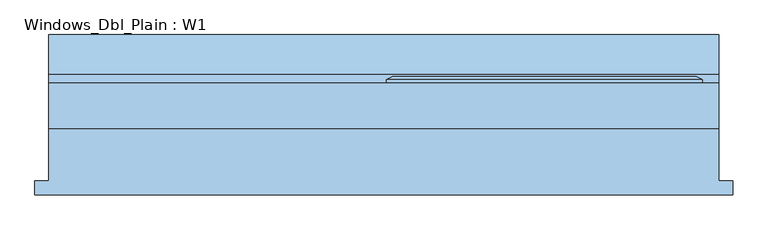
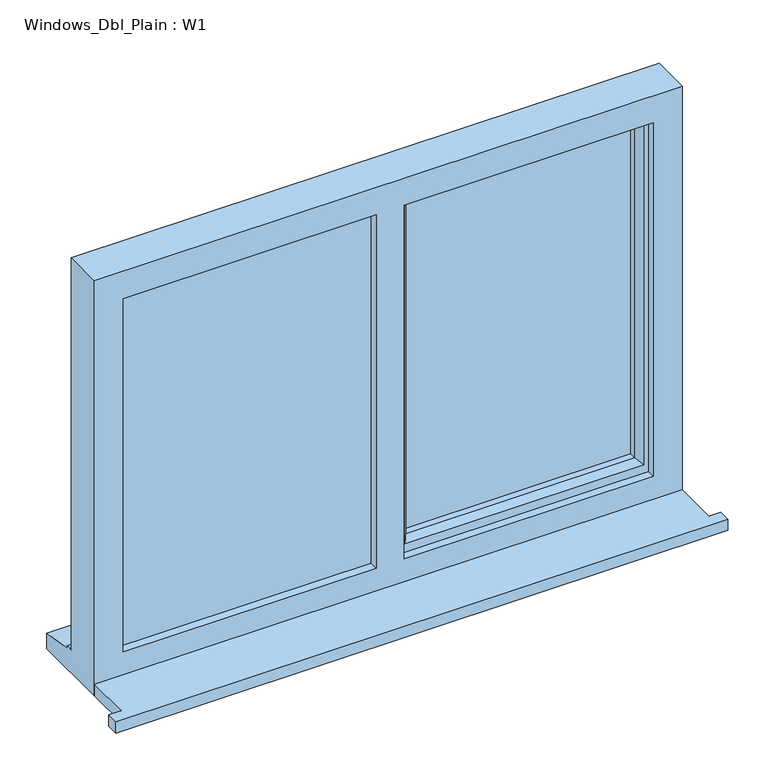
"""IFC4 building model written with IfcOpenShell, lengths in millimetres: window geometry, Windows_Dbl_Plain : W1."""

from ifc_helpers import new_model, si_unit, frame, origin, place, context, project, spatial, polyline, outline, extrude, faceted_brep, source, transform, mapped, element, save


def windows_dbl_plain_w1_9e0d93ab(model_context):
    return source(origin(), model_context, "Body", "SolidModel", [
        extrude(outline(polyline([(-919.6, -130.8434322), (-919.6, -105.8434322), (-894.6, -105.8434322), (-894.6, -10.2434322), (324.6, -10.2434322), (324.6, -105.8434322), (349.6, -105.8434322), (349.6, -130.8434322), (-919.6, -130.8434322)])), frame((0.0, 0.0, 1200.0), z_axis=(0.0, 0.0, 1.0), x_axis=(1.0, 0.0, 0.0)), (0.0, 0.0, 1.0), 25.0),
        faceted_brep([(-280.0, 72.7565678, 2080.0), (-280.0, 78.5300705, 2080.0), (-280.0, 78.5300705, 1253.0), (-280.0, 72.7565678, 1253.0), (-270.0, 7.7565678, 2070.0), (-270.0, 72.7565678, 2070.0), (-270.0, 72.7565678, 1263.0), (-270.0, 7.7565678, 1263.0), (-230.0, 22.2494677, 2030.0), (-240.1480377, 7.7565678, 2040.1480377), (-240.1480377, 7.7565678, 1292.8519623), (-230.0, 22.2494677, 1303.0), (-230.0, 36.7565678, 2030.0), (-230.0, 36.7565678, 1303.0), (-240.0, 60.7565678, 2040.0), (-240.0, 36.7565678, 2040.0), (-240.0, 36.7565678, 1293.0), (-240.0, 60.7565678, 1293.0), (-230.0, 78.5300705, 2030.0), (-230.0, 60.7565678, 2030.0), (-230.0, 60.7565678, 1303.0), (-230.0, 78.5300705, 1303.0), (-247.4457548, 84.3035732, 2047.4457548), (-247.4457548, 84.3035732, 1285.5542452), (-269.2153903, 84.3035732, 2069.2153903), (-269.2153903, 84.3035732, 1263.7846097), (294.6, 78.5300705, 1253.0), (294.6, 72.7565678, 1253.0), (284.6, 72.7565678, 1263.0), (284.6, 7.7565678, 1263.0), (254.7480377, 7.7565678, 1292.8519623), (244.6, 22.2494677, 1303.0), (244.6, 36.7565678, 1303.0), (254.6, 36.7565678, 1293.0), (254.6, 60.7565678, 1293.0), (244.6, 60.7565678, 1303.0), (244.6, 78.5300705, 1303.0), (262.0457548, 84.3035732, 1285.5542452), (283.8153903, 84.3035732, 1263.7846097), (294.6, 78.5300705, 2080.0), (294.6, 72.7565678, 2080.0), (284.6, 72.7565678, 2070.0), (284.6, 7.7565678, 2070.0), (254.7480377, 7.7565678, 2040.1480377), (244.6, 22.2494677, 2030.0), (244.6, 36.7565678, 2030.0), (254.6, 36.7565678, 2040.0), (254.6, 60.7565678, 2040.0), (244.6, 60.7565678, 2030.0), (244.6, 78.5300705, 2030.0), (262.0457548, 84.3035732, 2047.4457548), (283.8153903, 84.3035732, 2069.2153903)], [[[0, 1, 2, 3]], [[4, 5, 6, 7]], [[8, 9, 10, 11]], [[12, 8, 11, 13]], [[14, 15, 16, 17]], [[18, 19, 20, 21]], [[22, 18, 21, 23]], [[1, 24, 25, 2]], [[3, 2, 26, 27]], [[7, 6, 28, 29]], [[11, 10, 30, 31]], [[13, 11, 31, 32]], [[17, 16, 33, 34]], [[21, 20, 35, 36]], [[23, 21, 36, 37]], [[2, 25, 38, 26]], [[27, 26, 39, 40]], [[29, 28, 41, 42]], [[31, 30, 43, 44]], [[32, 31, 44, 45]], [[34, 33, 46, 47]], [[36, 35, 48, 49]], [[37, 36, 49, 50]], [[26, 38, 51, 39]], [[40, 39, 1, 0]], [[3, 27, 40, 0], [5, 41, 28, 6]], [[42, 41, 5, 4]], [[7, 29, 42, 4], [9, 43, 30, 10]], [[44, 43, 9, 8]], [[45, 44, 8, 12]], [[15, 46, 33, 16], [13, 32, 45, 12]], [[47, 46, 15, 14]], [[17, 34, 47, 14], [19, 48, 35, 20]], [[49, 48, 19, 18]], [[50, 49, 18, 22]], [[24, 51, 38, 25], [23, 37, 50, 22]], [[39, 51, 24, 1]]]),
        extrude(outline(polyline([(2050.0, -310.0), (2070.0, -310.0), (2070.0, -854.6), (1263.0, -854.6), (1263.0, -310.0), (1283.0, -310.0), (1283.0, -834.6), (2050.0, -834.6), (2050.0, -310.0)])), frame((0.0, 31.7565678, 0.0), z_axis=(0.0, 1.0, 0.0), x_axis=(0.0, 0.0, 1.0)), (0.0, 0.0, 1.0), 41.0),
        faceted_brep([(324.6, -10.2434322, 2110.0), (-894.6, -10.2434322, 2110.0), (-894.6, -10.2434322, 1200.0), (324.6, -10.2434322, 1200.0), (264.6, -10.2434322, 2050.0), (264.6, -10.2434322, 1275.0), (-252.0, -10.2434322, 1275.0), (-252.0, -10.2434322, 2050.0), (-310.0, -10.2434322, 2050.0), (-310.0, -10.2434322, 1275.0), (-834.6, -10.2434322, 1275.0), (-834.6, -10.2434322, 2050.0), (-894.6, 72.7565678, 2110.0), (-894.6, 72.7565678, 1251.0), (-894.6, 87.7565678, 1249.68767), (-894.6, 87.7565678, 1244.7449676), (-894.6, 160.2565678, 1233.8088847), (-894.6, 160.2565678, 1200.0), (324.6, 72.7565678, 2110.0), (324.6, 72.7565678, 1251.0), (-854.6, 72.7565678, 2070.0), (-854.6, 72.7565678, 1263.0), (-310.0, 72.7565678, 1263.0), (-310.0, 72.7565678, 2070.0), (-270.0, 72.7565678, 2070.0), (-270.0, 72.7565678, 1263.0), (284.6, 72.7565678, 1263.0), (284.6, 72.7565678, 2070.0), (-854.6, 7.7565678, 2070.0), (-854.6, 7.7565678, 1263.0), (-300.0, 7.7565678, 2070.0), (-300.0, 7.7565678, 1263.0), (-310.0, 7.7565678, 2050.0), (-834.6, 7.7565678, 2050.0), (-834.6, 7.7565678, 1275.0), (-310.0, 7.7565678, 1275.0), (-270.0, 7.7565678, 2070.0), (284.6, 7.7565678, 2070.0), (284.6, 7.7565678, 1263.0), (-270.0, 7.7565678, 1263.0), (264.6, 7.7565678, 2050.0), (-252.0, 7.7565678, 2050.0), (-252.0, 7.7565678, 1275.0), (264.6, 7.7565678, 1275.0), (-310.0, 31.7565678, 2070.0), (-300.0, 31.7565678, 2070.0), (324.6, 160.2565678, 1200.0), (324.6, 160.2565678, 1233.8088847), (324.6, 87.7565678, 1244.7449676), (324.6, 87.7565678, 1249.68767), (-300.0, 31.7565678, 1263.0), (-310.0, 31.7565678, 1263.0)], [[[0, 1, 2, 3], [4, 5, 6, 7], [8, 9, 10, 11]], [[2, 1, 12, 13, 14, 15, 16, 17]], [[13, 12, 18, 19], [20, 21, 22, 23], [24, 25, 26, 27]], [[21, 20, 28, 29]], [[28, 30, 31, 29], [32, 33, 34, 35]], [[36, 37, 38, 39], [40, 41, 42, 43]], [[33, 11, 10, 34]], [[1, 0, 18, 12]], [[28, 20, 23, 44, 45, 30]], [[27, 37, 36, 24]], [[11, 33, 32, 8]], [[40, 4, 7, 41]], [[19, 18, 0, 3, 46, 47, 48, 49]], [[27, 26, 38, 37]], [[4, 40, 43, 5]], [[45, 50, 31, 30]], [[50, 45, 44, 51]], [[51, 44, 23, 22]], [[25, 24, 36, 39]], [[41, 7, 6, 42]], [[8, 32, 35, 9]], [[46, 3, 2, 17]], [[47, 46, 17, 16]], [[48, 47, 16, 15]], [[49, 48, 15, 14]], [[19, 49, 14, 13]], [[22, 21, 29, 31, 50, 51]], [[26, 25, 39, 38]], [[6, 5, 43, 42]], [[35, 34, 10, 9]]]),
        extrude(outline(polyline([(-854.6, 31.7565678), (-300.0, 31.7565678), (-300.0, 7.7565678), (-854.6, 7.7565678), (-854.6, 31.7565678)])), frame((0.0, 0.0, 1263.0), z_axis=(0.0, 0.0, 1.0), x_axis=(1.0, 0.0, 0.0)), (0.0, 0.0, 1.0), 807.0),
        extrude(outline(polyline([(254.6, 36.7565678), (-240.0, 36.7565678), (-240.0, 60.7565678), (254.6, 60.7565678), (254.6, 36.7565678)])), frame((0.0, 0.0, 1293.0), z_axis=(0.0, 0.0, 1.0), x_axis=(1.0, 0.0, 0.0)), (0.0, 0.0, 1.0), 747.0),
    ])


if __name__ == "__main__":
    model = new_model("IFC4")
    model_context = context("Model", 3, world=origin())
    ifc_project = project(units=[si_unit("LENGTHUNIT", "METRE", prefix="MILLI")], contexts=[model_context])
    site = spatial("IfcSite", under=ifc_project)
    building = spatial("IfcBuilding", under=site)
    placement = place(None, origin())
    windows_dbl_plain_w1_shape = windows_dbl_plain_w1_9e0d93ab(model_context)
    element("IfcWindow", 1, ObjectType="Windows_Dbl_Plain : W1", at=placement, inside=building, context=model_context, shape_type="MappedRepresentation", body=[
        mapped(windows_dbl_plain_w1_shape, transform((0.0, 0.0, 0.0), x_axis=(1.0, 0.0, 0.0), y_axis=(0.0, 1.0, 0.0), z_axis=(0.0, 0.0, 1.0))),
    ])
    save(model, "model.ifc")

# Revit data of these elements
# Type "Windows_Dbl_Plain : W1"
#   Type Mark = "62"
#   Operation = "DoublePanelVertical"
#   Construction Type Id = "GSP4R"
#   Manufacturer = "Revit"
#   Keynote = "L10"
#   Analytic Construction = "1/8 in Pilkington single glazing"
#   Wrap Layers (Ext) from Ext = 0.336286 ft
#   Wrap Layers (Int) from Ext = 0.582349 ft
#   Window Board Projection = 0.082021 ft
#   Window Board Extension = 0.082021 ft
#   Visual Light Transmittance = 0.9
#   Solar Heat Gain Coefficient = 0.78
#   Rough Width = 4.0 ft
#   Rough Height = 2.985564 ft
#   Height = 2.985564 ft
#   Width = 4.0 ft
#   Heat Transfer Coefficient (U) = 3.6886 W/(m²·K)
#   Glazing Thickness = 0.07874 ft
#   FrameOffset - External = 0.164042 ft
#   Frame Depth = 0.213255 ft
#   Default Head Height = 6.922572 ft
#   Cill Depth = 0.287073 ft
#   Cavity Closer Width = 0.164042 ft
#   Cavity Closer Offset from Ext = 0.336286 ft
#   Cavity Closer Depth = 0.278871 ft
#   Vis - Cavity Closers = yes
#   Define Thermal Properties by = 1
#   Material Trim = Window Frame
#   Material Glass = Glass
#   Material Frame = Cherry
#   Wall Closure = (empty or 0)
# Element 1 (IfcWindow, "Windows_Dbl_Plain : W1")
#   Materials on its faces: "Cherry", "Glass", "Window Frame"
# Materials
#   "Window Frame": colour RGB 249 249 249, transparency 0, Keynote = "L10", Cost = 0
#   "Glass": class "Glass", colour RGB 0 128 192, transparency 0.9, Description = "Soda Lime Glass", Cost = 0
#   "Cherry": class "Wood", colour RGB 226 177 128, transparency 0, Description = "Prunus Serotina", Cost = 0
